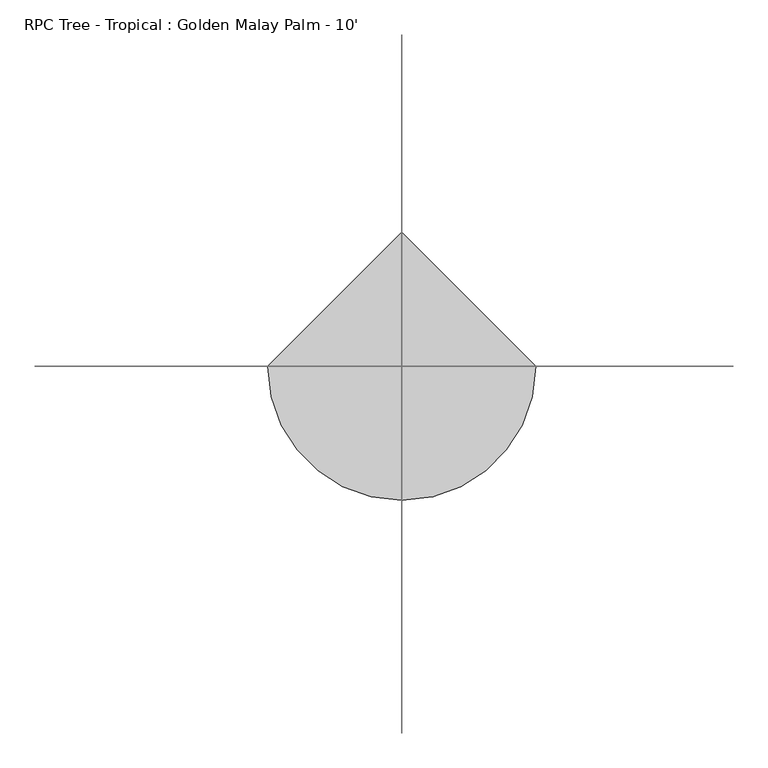
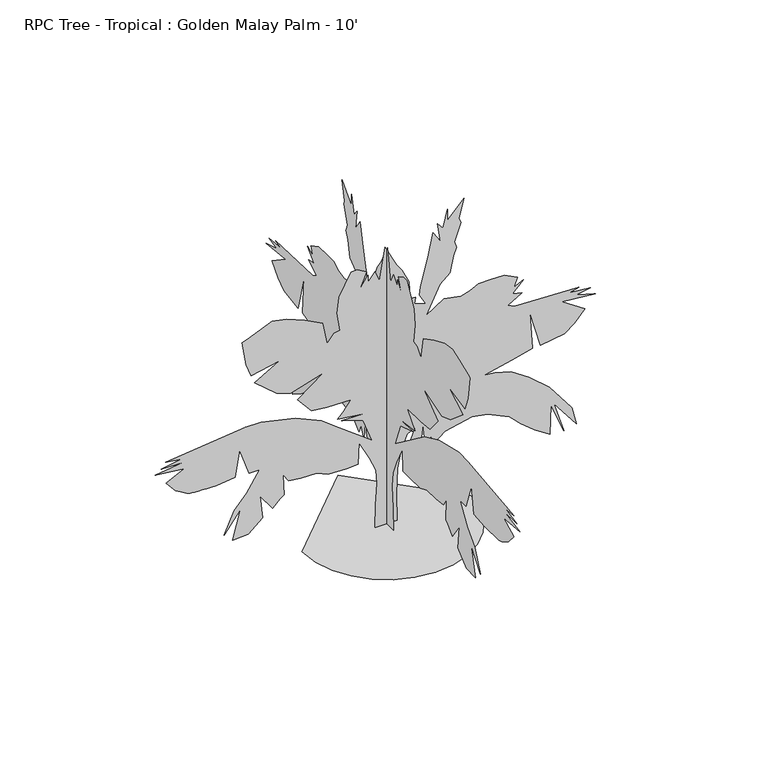
"""IFC4 building model written with IfcOpenShell, lengths in millimetres: geographic element geometry, RPC Tree - Tropical : Golden Malay Palm - 10'."""

from ifc_helpers import new_model, si_unit, origin, place, context, project, spatial, triangles, source, transform, mapped, element, save


def rpc_tree_tropical_golden_malay_palm_10_a310d7cf(model_context):
    return source(origin(), model_context, "Body", "Tessellation", [
        triangles([(9.89e-05, 133.5213922, 670.0644053), (0.0001158, 103.2936315, 529.0005229), (0.0001458, 93.2174569, 277.101182), (0.0001788, 98.2555397, 0.010878), (0.0001788, -113.3400931, 0.010878), (0.0001518, -108.30251, 226.7208087), (0.000126, -93.1884979, 443.3542972), (0.0001098, -103.2644181, 579.3813867), (9.23e-05, -163.7202029, 725.4820982), (6.95e-05, -264.479932, 916.9269533), (9.53e-05, -274.5561157, 700.292938), (9.59e-05, -385.3915197, 695.2536381), (9.53e-05, -561.7207641, 700.292938), (8.93e-05, -672.5587297, 750.671331), (8.93e-05, -828.7356068, 750.671331), (8.75e-05, -944.6103653, 765.7868328), (7.79e-05, -994.9887583, 846.3936859), (0.0001026, -984.9125565, 639.8358725), (0.0001056, -1025.2172184, 614.6467123), (0.0001146, -1095.7504858, 539.0766884), (9.47e-05, -1216.6620735, 705.3297672), (0.0001218, -1191.4703699, 478.6196228), (0.0001362, -1332.536832, 357.7080714), (0.0001368, -1483.6744091, 352.6712422), (0.0001026, -1403.067556, 639.8358725), (0.0001272, -1564.283733, 433.2780953), (0.000102, -1468.5613781, 644.8752451), (8.57e-05, -1347.6498631, 780.8998638), (6.23e-05, -1221.69883, 977.3814754), (6.23e-05, -1322.4607029, 977.3814754), (3.11e-05, -1413.1436852, 1239.3569092), (6.17e-05, -1458.4852489, 982.4207754), (6.41e-05, -1639.8538296, 962.2684444), (6.4e-05, -1687.1180958, 963.3555874), (6.38e-05, -1732.9753258, 964.4858963), (6.37e-05, -1776.0104897, 965.7050806), (6.35e-05, -1814.8165512, 967.0563789), (6.34e-05, -1847.9838581, 968.5828846), (6.32e-05, -1874.0976711, 970.3329231), (6.29e-05, -1891.7531342, 972.3446463), (6.24e-05, -1906.0304604, 976.2663546), (6.16e-05, -1922.6852577, 983.3606163), (6.04e-05, -1941.3262711, 993.0989754), (5.9e-05, -1961.5497459, 1004.9505775), (5.74e-05, -1982.9670433, 1018.3922716), (5.57e-05, -2005.1742634, 1032.8880438), (5.39e-05, -2027.7802963, 1047.9146702), (4.13e-05, -2118.4632786, 1153.7132269), (3.11e-05, -1947.1708271, 1239.3569092), (2.75e-05, -2224.261908, 1269.585442), (2.27e-05, -1952.2101997, 1309.8901039), (2.21e-05, -2168.844215, 1314.9270058), (1.79e-05, -1977.3993599, 1350.1949112), (1.55e-05, -2123.5001804, 1370.3471695), (5.3e-06, -1357.7259922, 1455.9909245), (5.3e-06, -1206.5858717, 1455.9909245), (1.43e-05, -874.0771706, 1380.4208279), (2.81e-05, -627.2171659, 1264.5486855), (4.37e-05, -455.9247508, 1133.5608959), (7.19e-05, -138.5302706, 896.7745497), (4.37e-05, -229.2143339, 1133.5608959), (3.59e-05, -435.7723835, 1199.0547907), (3.65e-05, -219.1381502, 1194.0154181), (3.23e-05, -471.0377455, 1229.2832508), (2.63e-05, -420.6568454, 1279.6617165), (1.43e-05, -340.0499923, 1380.4208279), (1.37e-05, -571.7995093, 1385.4602005), (1.19e-05, -722.9370501, 1400.5732315), (-7.4e-06, -858.9641396, 1561.7895538), (-2.96e-05, -607.064835, 1748.194891), (-1.82e-05, -924.4580343, 1652.4750069), (-2.36e-05, -1060.4851238, 1697.8165707), (-4.52e-05, -1272.0797665, 1879.1826805), (-6.14e-05, -1030.256591, 2015.2098427), (-5.48e-05, -1302.3082993, 1959.7921497), (-7.04e-05, -1352.6890903, 2090.7797939), (-9.86e-05, -1387.954525, 2327.5662128), (-9.98e-05, -1352.6890903, 2337.642342), (-0.000107, -1211.6227009, 2398.0967915), (-0.0001125, -1100.787315, 2443.4383553), (-0.0001095, -964.7627689, 2418.2491951), (-0.0001004, -788.4309448, 2342.6790985), (-8.96e-05, -617.1410368, 2251.9961163), (-6.32e-05, -571.7995093, 2030.3227283), (-7.28e-05, -506.3030711, 2110.9321976), (-7.4e-05, -445.848549, 2121.0083267), (-9.62e-05, -476.0770818, 2307.4138092), (-0.0001149, -455.9247508, 2463.5906136), (-0.0001401, -340.0499923, 2675.1776985), (-0.0001407, -284.6322812, 2680.2323318), (-0.0001347, -193.9479727, 2629.8386055), (-0.0001155, -259.443121, 2468.6301315), (-0.0001299, -178.834215, 2589.5288567), (-0.0001215, -178.834215, 2519.0084518), (-0.0001311, -113.3400931, 2599.6128342), (-0.0001185, -67.9985656, 2493.8192917), (-0.0001569, -17.6182708, 2816.2493202), (-0.0001311, 93.2174569, 2599.6128342), (-0.0001221, 148.6356586, 2524.0476791), (-0.0001052, 214.1292808, 2382.9839058), (-8.42e-05, 224.2057188, 2206.6545525), (-8.42e-05, 279.6234118, 2206.6545525), (-7.64e-05, 269.5472281, 2141.1607304), (-7.16e-05, 380.3826322, 2100.8560684), (-8.48e-05, 314.8887374, 2211.6914543), (-9.5e-05, 324.9649392, 2297.3376801), (-0.0001275, 395.4981703, 2569.3867722), (-0.0001551, 445.8764906, 2801.1362892), (-0.0001419, 516.4097217, 2690.2907295), (-0.0001641, 491.2205615, 2876.7011536), (-0.0001563, 541.5989182, 2811.219976), (-0.0001779, 586.9404093, 2992.5760574), (-0.0001641, 586.9404093, 2876.7011536), (-0.0001845, 743.1199024, 3047.9988373), (-0.0001623, 697.7783386, 2861.5881226), (-0.0001569, 712.8913696, 2816.2493202), (-0.0001359, 652.434304, 2639.922583), (-0.0001281, 672.586635, 2574.4158257), (-0.0001191, 642.3581022, 2498.8561935), (-9.98e-05, 607.0927766, 2337.642342), (-9.02e-05, 511.3703854, 2257.0328728), (-5.72e-05, 380.3826322, 1979.944408), (-7.1e-05, 551.6750836, 2095.8166958), (-6.68e-05, 712.8913696, 2060.5512611), (-6.98e-05, 803.5744246, 2085.7404213), (-7.52e-05, 884.1838211, 2131.0846012), (-7.52e-05, 995.019207, 2131.0846012), (-7.52e-05, 1131.0462965, 2131.0846012), (-6.74e-05, 1256.9946407, 2065.5906338), (-5.66e-05, 1226.7661079, 1974.9050354), (-6.2e-05, 1317.4517063, 2020.2465992), (-4.94e-05, 1211.6531496, 1914.4505859), (-4.7e-05, 1302.3362045, 1894.2981823), (-3.74e-05, 1166.3116585, 1813.6888584), (-3.32e-05, 1231.8054806, 1778.4234238), (-3.02e-05, 1851.4788483, 1753.2342636), (-2.78e-05, 1755.7564934, 1733.0820053), (-2.54e-05, 1962.3143795, 1712.9296017), (-2.24e-05, 1826.2896881, 1687.7404415), (-1.58e-05, 2007.655798, 1632.3227486), (-2e-05, 1685.2257694, 1667.5880379), (-1.9e-06, 1906.8966866, 1516.44799), (1.13e-05, 1806.1374298, 1405.6126041), (2.03e-05, 1710.4149296, 1330.0425076), (2.45e-05, 1478.6680286, 1294.7772182), (-1.94e-05, 1377.9063011, 1662.5486652), (2.45e-05, 1403.0979321, 1294.7772182), (3.05e-05, 1211.6531496, 1244.3962818), (3.77e-05, 934.5621414, 1183.9392162), (3.95e-05, 1040.3606981, 1168.8262579), (4.43e-05, 1196.5401913, 1128.5215233), (5.81e-05, 1367.8300266, 1012.6493082), (7.85e-05, 1564.3117836, 841.3568567), (0.0001128, 1780.9482697, 554.1896831), (0.0001338, 1826.2896881, 377.8604024), (0.0001007, 1609.6558182, 654.9514469), (0.0001374, 1705.3781731, 347.6318696), (0.0001014, 1579.4272854, 649.9120743), (0.0001356, 1569.3510109, 362.7474077), (0.0001242, 1423.2503357, 458.4697989), (0.0001116, 1292.2600754, 564.2658485), (9.83e-05, 1181.4246168, 675.1012344), (8.63e-05, 969.8300468, 775.8630346), (8.33e-05, 818.6899263, 801.0521948), (8.99e-05, 561.7512491, 745.6345018), (0.0001001, 455.9526924, 659.9882761), (9.05e-05, 425.7267031, 740.5976727), (0.0001032, 380.3826322, 634.7991159), (7.43e-05, 350.1566428, 876.6222187), (9.71e-05, 324.9649392, 685.1774363), (9.89e-05, 234.2813756, 670.0644053), (8.63e-05, 234.2813756, 775.8630346), (7.31e-05, 279.6234118, 886.6984205), (7.85e-05, 193.9774404, 841.3568567), (8.87e-05, 163.7496706, 755.710631), (133.5213922, 0.0001645, 670.0644053), (103.2936315, 0.0001813, 529.0005229), (93.2174569, 0.0002114, 277.101182), (98.2555397, 0.0002444, 0.0107758), (-113.3400931, 0.0002444, 0.0108645), (-108.30251, 0.0002174, 226.7208087), (-93.1887523, 0.0001915, 443.3542972), (-103.2644181, 0.0001753, 579.3813867), (-163.7204573, 0.0001579, 725.4820982), (-264.479932, 0.0001351, 916.9269533), (-274.5561157, 0.0001609, 700.292938), (-385.3915197, 0.0001615, 695.2536381), (-561.7233075, 0.0001609, 700.292938), (-672.5587297, 0.0001549, 750.671331), (-828.7356068, 0.0001549, 750.671331), (-944.6103653, 0.0001531, 765.7868328), (-994.9912291, 0.0001435, 846.3936859), (-984.9125565, 0.0001681, 639.8358725), (-1025.2172184, 0.0001711, 614.6467123), (-1095.7504858, 0.0001801, 539.0766884), (-1216.6620735, 0.0001603, 705.3297672), (-1191.4703699, 0.0001873, 478.6196228), (-1332.536832, 0.0002018, 357.7080714), (-1483.6744091, 0.0002024, 352.6712422), (-1403.067556, 0.0001681, 639.8358725), (-1564.283733, 0.0001927, 433.2780953), (-1468.5613781, 0.0001675, 644.8752451), (-1347.6498631, 0.0001513, 780.8998638), (-1221.69883, 0.0001279, 977.3814754), (-1322.4607029, 0.0001279, 977.3814754), (-1413.1436852, 9.67e-05, 1239.3569092), (-1458.4852489, 0.0001273, 982.4207754), (-1639.8538296, 0.0001297, 962.2684444), (-1687.1180958, 0.0001296, 963.3555874), (-1732.9753258, 0.0001294, 964.4858963), (-1776.0104897, 0.0001293, 965.7050806), (-1814.8165512, 0.0001291, 967.0563789), (-1847.9838581, 0.0001289, 968.5828846), (-1874.0976711, 0.0001287, 970.3329231), (-1891.7531342, 0.0001285, 972.3446463), (-1906.0304604, 0.000128, 976.2663546), (-1922.6852577, 0.0001272, 983.3606163), (-1941.3262711, 0.000126, 993.0989754), (-1961.5497459, 0.0001246, 1004.9505775), (-1982.9670433, 0.000123, 1018.3922716), (-2005.1742634, 0.0001213, 1032.8880438), (-2027.7802963, 0.0001195, 1047.9146702), (-2118.4632786, 0.0001069, 1153.7132269), (-1947.1708271, 9.67e-05, 1239.3569092), (-2224.261908, 9.31e-05, 1269.585442), (-1952.2101997, 8.82e-05, 1309.8901039), (-2168.844215, 8.76e-05, 1314.9270058), (-1977.3993599, 8.34e-05, 1350.1949112), (-2123.5001804, 8.1e-05, 1370.3471695), (-1357.7259922, 7.08e-05, 1455.9909245), (-1206.5858717, 7.08e-05, 1455.9909245), (-874.0771706, 7.98e-05, 1380.4208279), (-627.2171659, 9.37e-05, 1264.5486855), (-455.9247508, 0.0001093, 1133.5608959), (-138.5302706, 0.0001375, 896.7745497), (-229.2145882, 0.0001093, 1133.5608959), (-435.7723835, 0.0001015, 1199.0547907), (-219.1381502, 0.0001021, 1194.0154181), (-471.0377455, 9.79e-05, 1229.2832508), (-420.6593888, 9.18e-05, 1279.6617165), (-340.0499923, 7.98e-05, 1380.4208279), (-571.7995093, 7.92e-05, 1385.4602005), (-722.9370501, 7.74e-05, 1400.5732315), (-858.9641396, 5.82e-05, 1561.7895538), (-607.064835, 3.6e-05, 1748.194891), (-924.4580343, 4.74e-05, 1652.4750069), (-1060.4851238, 4.2e-05, 1697.8165707), (-1272.0797665, 2.04e-05, 1879.1826805), (-1030.256591, 4.2e-06, 2015.2098427), (-1302.3082993, 1.08e-05, 1959.7921497), (-1352.6890903, -4.8e-06, 2090.7797939), (-1387.954525, -3.31e-05, 2327.5662128), (-1352.6890903, -3.43e-05, 2337.642342), (-1211.6227009, -4.15e-05, 2398.0967915), (-1100.787315, -4.69e-05, 2443.4383553), (-964.7627689, -4.39e-05, 2418.2491951), (-788.4309448, -3.49e-05, 2342.6790985), (-617.1410368, -2.41e-05, 2251.9961163), (-571.7995093, 2.4e-06, 2030.3227283), (-506.3030711, -7.2e-06, 2110.9321976), (-445.848549, -8.4e-06, 2121.0083267), (-476.0770818, -3.07e-05, 2307.4138092), (-455.9247508, -4.93e-05, 2463.5906136), (-340.0499923, -7.45e-05, 2675.1776985), (-284.6322812, -7.51e-05, 2680.2323318), (-193.948227, -6.91e-05, 2629.8386055), (-259.443121, -4.99e-05, 2468.6301315), (-178.834215, -6.43e-05, 2589.5288567), (-178.834215, -5.59e-05, 2519.0084518), (-113.3400931, -6.55e-05, 2599.6128342), (-67.9985656, -5.29e-05, 2493.8192917), (-17.6183468, -9.13e-05, 2816.2493202), (93.2174569, -6.55e-05, 2599.6128342), (148.6356586, -5.65e-05, 2524.0476791), (214.1292808, -3.97e-05, 2382.9839058), (224.2054645, -1.87e-05, 2206.6545525), (279.6234118, -1.87e-05, 2206.6545525), (269.5472281, -1.08e-05, 2141.1607304), (380.3826322, -6e-06, 2100.8560684), (314.8887374, -1.93e-05, 2211.6914543), (324.9649392, -2.95e-05, 2297.3376801), (395.4981703, -6.19e-05, 2569.3867722), (445.8764906, -8.95e-05, 2801.1362892), (516.4097217, -7.63e-05, 2690.2907295), (491.2205615, -9.85e-05, 2876.7011536), (541.5989182, -9.07e-05, 2811.219976), (586.9404093, -0.0001123, 2992.5760574), (586.9404093, -9.85e-05, 2876.7011536), (743.1199024, -0.000119, 3047.9988373), (697.7757952, -9.67e-05, 2861.5881226), (712.8913696, -9.13e-05, 2816.2493202), (652.434304, -7.03e-05, 2639.922583), (672.586635, -6.25e-05, 2574.4158257), (642.3581022, -5.35e-05, 2498.8561935), (607.0927766, -3.43e-05, 2337.642342), (511.3703854, -2.47e-05, 2257.0328728), (380.3826322, 8.4e-06, 1979.944408), (551.6750836, -5.4e-06, 2095.8166958), (712.8913696, -1.2e-06, 2060.5512611), (803.5744246, -4.2e-06, 2085.7404213), (884.1838211, -9.6e-06, 2131.0846012), (995.019207, -9.6e-06, 2131.0846012), (1131.0462965, -9.6e-06, 2131.0846012), (1256.9946407, -1.8e-06, 2065.5906338), (1226.7661079, 9e-06, 1974.9050354), (1317.4517063, 3.6e-06, 2020.2465992), (1211.6531496, 1.62e-05, 1914.4505859), (1302.3362045, 1.86e-05, 1894.2981823), (1166.3116585, 2.82e-05, 1813.6888584), (1231.8054806, 3.24e-05, 1778.4234238), (1851.4788483, 3.54e-05, 1753.2342636), (1755.7564934, 3.78e-05, 1733.0820053), (1962.3143795, 4.02e-05, 1712.9296017), (1826.2896881, 4.32e-05, 1687.7404415), (2007.655798, 4.98e-05, 1632.3227486), (1685.2232986, 4.56e-05, 1667.5880379), (1906.8966866, 6.36e-05, 1516.44799), (1806.1374298, 7.68e-05, 1405.6126041), (1710.4149296, 8.58e-05, 1330.0425076), (1478.6680286, 9e-05, 1294.7772182), (1377.9063011, 4.62e-05, 1662.5486652), (1403.0954613, 9e-05, 1294.7772182), (1211.6531496, 9.61e-05, 1244.3962818), (934.5621414, 0.0001033, 1183.9392162), (1040.3606981, 0.0001051, 1168.8262579), (1196.5401913, 0.0001099, 1128.5215233), (1367.8300266, 0.0001237, 1012.6493082), (1564.3117836, 0.0001441, 841.3568567), (1780.9456535, 0.0001783, 554.1896831), (1826.2896881, 0.0001994, 377.8604024), (1609.6558182, 0.0001663, 654.9514469), (1705.3757023, 0.000203, 347.6318696), (1579.4272854, 0.0001669, 649.9120743), (1569.3510109, 0.0002012, 362.7474077), (1423.2503357, 0.0001897, 458.4672918), (1292.2600754, 0.0001771, 564.2658485), (1181.4246168, 0.0001639, 675.1012344), (969.8300468, 0.0001519, 775.8630346), (818.6899263, 0.0001489, 801.0521948), (561.7512491, 0.0001555, 745.6345018), (455.9526924, 0.0001657, 659.9882761), (425.7241596, 0.0001561, 740.5951292), (380.3826322, 0.0001687, 634.7991159), (350.1566428, 0.0001399, 876.6222187), (324.9649392, 0.0001627, 685.1774363), (234.2813756, 0.0001645, 670.0644053), (234.2813756, 0.0001519, 775.8630346), (279.6234118, 0.0001387, 886.6984205), (193.9774404, 0.0001441, 841.3568567), (163.7496706, 0.0001543, 755.710631), (-812.451717, 0.0, 7.05e-05), (-790.9734495, -186.160076, 7.3e-05), (-729.802692, -357.1187905, 8.03e-05), (-633.8364567, -507.9769515, 9.18e-05), (-507.9769515, -633.8364567, 0.0001068), (-357.1187905, -729.802692, 1.08e-05), (-186.1598216, -790.9734495, 3.12e-05), (3.55e-05, -812.451717, 5.34e-05), (186.160076, -790.9734495, 7.56e-05), (357.1187905, -729.802692, 9.6e-05), (507.9769515, -633.8364567, 0.0), (633.8364567, -507.9769515, 1.5e-05), (729.802692, -357.1187905, 2.64e-05), (790.9734495, -186.1598216, 3.37e-05), (812.451717, 7.1e-05, 3.63e-05), (-0.0001065, 812.451717, 5.34e-05)], [[157, 156, 158], [140, 139, 141], [52, 51, 53], [26, 25, 27], [112, 111, 113], [136, 135, 137], [54, 53, 55], [50, 49, 51], [138, 137, 139], [62, 61, 63], [131, 130, 132], [155, 154, 156], [154, 153, 156], [114, 113, 115], [110, 109, 111], [168, 167, 169], [93, 92, 94], [97, 96, 98], [139, 137, 141], [133, 132, 134], [108, 107, 109], [137, 135, 141], [27, 25, 28], [64, 63, 65], [159, 158, 160], [95, 94, 96], [53, 51, 55], [73, 72, 74], [166, 165, 167], [24, 23, 25], [23, 22, 25], [22, 21, 25], [25, 21, 28], [65, 63, 66], [48, 47, 49], [20, 19, 21], [171, 170, 172], [170, 169, 172], [172, 169, 173], [102, 101, 103], [142, 141, 143], [156, 153, 158], [69, 68, 70], [68, 67, 70], [28, 21, 29], [5, 4, 6], [4, 3, 6], [6, 3, 7], [3, 2, 7], [7, 2, 8], [2, 1, 8], [160, 158, 161], [8, 1, 9], [98, 96, 99], [11, 10, 12], [145, 144, 146], [144, 143, 146], [143, 141, 146], [141, 135, 146], [67, 66, 70], [91, 90, 92], [90, 89, 92], [89, 88, 92], [77, 76, 78], [88, 87, 92], [1, 175, 9], [129, 128, 130], [75, 74, 76], [51, 49, 55], [47, 46, 49], [147, 146, 148], [158, 153, 161], [153, 152, 161], [161, 152, 162], [162, 152, 163], [152, 151, 163], [151, 150, 163], [150, 149, 163], [163, 149, 164], [72, 71, 74], [71, 70, 74], [76, 74, 78], [78, 74, 79], [79, 74, 80], [80, 74, 81], [81, 74, 82], [74, 70, 82], [82, 70, 83], [83, 70, 84], [32, 31, 33], [146, 135, 148], [148, 135, 149], [135, 134, 149], [99, 96, 100], [46, 45, 49], [30, 29, 31], [9, 175, 10], [175, 174, 10], [45, 44, 49], [49, 44, 55], [44, 43, 55], [43, 42, 55], [42, 41, 55], [41, 40, 55], [40, 39, 55], [39, 38, 55], [38, 37, 55], [37, 36, 55], [36, 35, 55], [35, 34, 55], [34, 33, 55], [33, 31, 55], [55, 31, 56], [31, 29, 56], [56, 29, 57], [57, 29, 58], [100, 96, 101], [29, 21, 58], [115, 113, 116], [116, 113, 117], [113, 111, 117], [111, 109, 117], [109, 107, 117], [117, 107, 118], [118, 107, 119], [107, 106, 119], [119, 106, 120], [120, 106, 121], [106, 105, 121], [105, 104, 121], [121, 104, 122], [104, 103, 122], [167, 165, 169], [12, 10, 13], [87, 86, 92], [164, 149, 165], [165, 149, 169], [18, 17, 19], [19, 17, 21], [21, 17, 58], [58, 17, 59], [17, 16, 59], [16, 15, 59], [15, 14, 59], [14, 13, 59], [13, 10, 59], [59, 10, 60], [10, 174, 60], [60, 174, 61], [61, 174, 63], [174, 173, 63], [128, 127, 130], [130, 127, 132], [132, 127, 134], [127, 126, 134], [126, 125, 134], [134, 125, 149], [125, 124, 149], [149, 124, 169], [124, 123, 169], [123, 122, 169], [169, 122, 173], [173, 122, 63], [63, 122, 66], [66, 122, 70], [122, 103, 70], [70, 103, 84], [84, 103, 85], [85, 103, 86], [103, 101, 86], [101, 96, 86], [86, 96, 92], [96, 94, 92], [331, 332, 333], [314, 315, 316], [226, 227, 228], [200, 201, 202], [286, 287, 288], [310, 311, 312], [228, 229, 230], [224, 225, 226], [312, 313, 314], [236, 237, 238], [305, 306, 307], [329, 330, 331], [328, 329, 331], [288, 289, 290], [284, 285, 286], [342, 343, 344], [267, 268, 269], [271, 272, 273], [312, 314, 316], [307, 308, 309], [282, 283, 284], [310, 312, 316], [200, 202, 203], [238, 239, 240], [333, 334, 335], [269, 270, 271], [226, 228, 230], [247, 248, 249], [340, 341, 342], [198, 199, 200], [197, 198, 200], [196, 197, 200], [196, 200, 203], [238, 240, 241], [222, 223, 224], [194, 195, 196], [345, 346, 347], [344, 345, 347], [344, 347, 348], [276, 277, 278], [316, 317, 318], [328, 331, 333], [243, 244, 245], [242, 243, 245], [196, 203, 204], [179, 180, 181], [178, 179, 181], [178, 181, 182], [177, 178, 182], [177, 182, 183], [176, 177, 183], [333, 335, 336], [176, 183, 184], [271, 273, 274], [185, 186, 187], [319, 320, 321], [318, 319, 321], [316, 318, 321], [310, 316, 321], [241, 242, 245], [265, 266, 267], [264, 265, 267], [263, 264, 267], [251, 252, 253], [262, 263, 267], [350, 176, 184], [303, 304, 305], [249, 250, 251], [224, 226, 230], [221, 222, 224], [321, 322, 323], [328, 333, 336], [327, 328, 336], [327, 336, 337], [327, 337, 338], [326, 327, 338], [325, 326, 338], [324, 325, 338], [324, 338, 339], [246, 247, 249], [245, 246, 249], [249, 251, 253], [249, 253, 254], [249, 254, 255], [249, 255, 256], [249, 256, 257], [245, 249, 257], [245, 257, 258], [245, 258, 259], [206, 207, 208], [310, 321, 323], [310, 323, 324], [309, 310, 324], [271, 274, 275], [220, 221, 224], [204, 205, 206], [350, 184, 185], [349, 350, 185], [219, 220, 224], [219, 224, 230], [218, 219, 230], [217, 218, 230], [216, 217, 230], [215, 216, 230], [214, 215, 230], [213, 214, 230], [212, 213, 230], [211, 212, 230], [210, 211, 230], [209, 210, 230], [208, 209, 230], [206, 208, 230], [206, 230, 231], [204, 206, 231], [204, 231, 232], [204, 232, 233], [271, 275, 276], [196, 204, 233], [288, 290, 291], [288, 291, 292], [286, 288, 292], [284, 286, 292], [282, 284, 292], [282, 292, 293], [282, 293, 294], [281, 282, 294], [281, 294, 295], [281, 295, 296], [280, 281, 296], [279, 280, 296], [279, 296, 297], [278, 279, 297], [340, 342, 344], [185, 187, 188], [261, 262, 267], [324, 339, 340], [324, 340, 344], [192, 193, 194], [192, 194, 196], [192, 196, 233], [192, 233, 234], [191, 192, 234], [190, 191, 234], [189, 190, 234], [188, 189, 234], [185, 188, 234], [185, 234, 235], [349, 185, 235], [349, 235, 236], [349, 236, 238], [348, 349, 238], [302, 303, 305], [302, 305, 307], [302, 307, 309], [301, 302, 309], [300, 301, 309], [300, 309, 324], [299, 300, 324], [299, 324, 344], [298, 299, 344], [297, 298, 344], [297, 344, 348], [297, 348, 238], [297, 238, 241], [297, 241, 245], [278, 297, 245], [278, 245, 259], [278, 259, 260], [278, 260, 261], [276, 278, 261], [271, 276, 261], [271, 261, 267], [269, 271, 267], [365, 366, 351], [364, 365, 351], [364, 351, 352], [363, 364, 352], [363, 352, 353], [363, 353, 354], [362, 363, 354], [361, 362, 354], [361, 354, 355], [361, 355, 356], [361, 356, 357], [361, 357, 358], [361, 358, 359], [361, 359, 360]], closed=False),
    ])


if __name__ == "__main__":
    model = new_model("IFC4")
    model_context = context("Model", 3, world=origin())
    ifc_project = project(units=[si_unit("LENGTHUNIT", "METRE", prefix="MILLI")], contexts=[model_context])
    site = spatial("IfcSite", under=ifc_project)
    building = spatial("IfcBuilding", under=site)
    placement = place(None, origin())
    rpc_tree_tropical_golden_malay_palm_10_shape = rpc_tree_tropical_golden_malay_palm_10_a310d7cf(model_context)
    element("IfcGeographicElement", 1, ObjectType="RPC Tree - Tropical : Golden Malay Palm - 10'", at=placement, inside=building, context=model_context, shape_type="MappedRepresentation", body=[
        mapped(rpc_tree_tropical_golden_malay_palm_10_shape, transform((0.0, 0.0, 0.0), x_axis=(1.0, 0.0, 0.0), y_axis=(0.0, 1.0, 0.0), z_axis=(0.0, 0.0, 1.0))),
    ])
    save(model, "model.ifc")

# Revit data of these elements
# Type "RPC Tree - Tropical : Golden Malay Palm - 10'"
#   built-in parameter 1005198 = "{2, 15},{39, RPC-16-FXGM-2RXX-PGXL-E000-ST1L-LVER-AU},{1, 0},{1, 0},{2, 13},{1, 8},{5, Color},{1, 0},{1, 0},{3, 0.8},{3, 0.8},{3, 0.8},{1, 8},{7, BBoxMin},{1, 0},{1, 0},{1, 0},{1, 0},{1, 0},{1, 8},{7, BBoxMax},{1, 0},{1, 0},{1, 0},{1, 0},{1, 0},{2, 11},{9, RPCTypeId},{1, 0},{1, 0},{39, RPC-16-FXGM-2RXX-PGXL-E000-ST1L-LVER-AU},{1, 6},{14, RPCPlantHeight},{1, 0},{1, 0},{2, 10},{2, 11},{7, keyword},{1, 0},{1, 0},{35, :RPCs:Trees [Tropical]:Geometry:RPC},{2, 11},{8, category},{1, 0},{1, 0},{16, Trees [Tropical]},{2, 11},{12, LocalizedUID},{1, 0},{1, 0},{17, Golden Malay Palm},{2, 14},{6, Height},{1, 0},{1, 0},{2, 10},{1, 2},{16, Cast Reflections},{1, 0},{1, 0},{1, 0},{1, 2},{12, Cast Shadows},{1, 0},{1, 0},{1, 1},{1, 2},{9, Lock View},{1, 0},{1, 0},{1, 0},{1, 4},{5, ViewC},{1, 0},{1, 0},{1, 0},{21, assetlibrary_base.fbx},{1, 5},"
#   built-in parameter 1005195 = "RPC-16-FXGM-2RXX-PGXL-E000-ST1L-LVER-AU"
#   Type Comments = "Golden Malay Palm"
#   Assembly Code = "G2050500"
#   Height = 10' - 0"
#   Plan Symbol = element 387627
#   Default Elevation = 0
